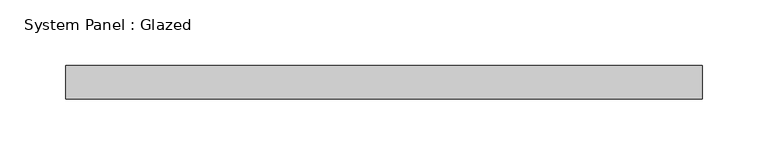
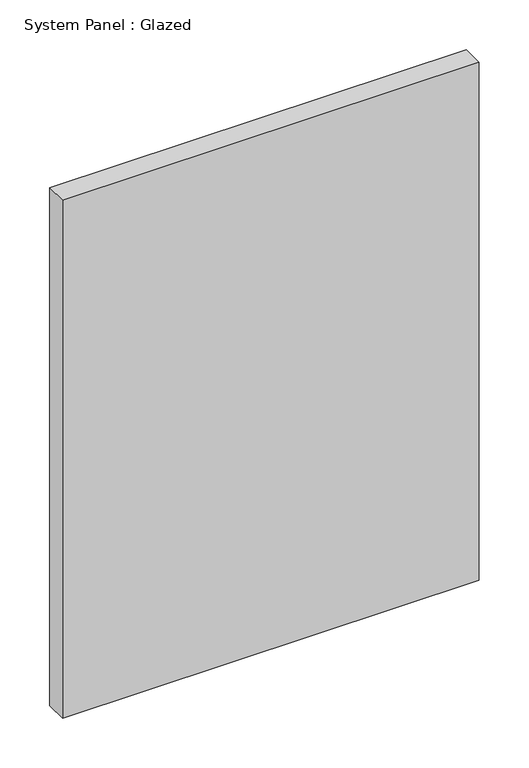
"""IFC4 building model written with IfcOpenShell, lengths in millimetres: plate geometry, System Panel : Glazed."""

from ifc_helpers import new_model, si_unit, origin, origin_with_axes, place, context, project, spatial, polyline, outline, extrude, source, transform, mapped, element, save


def system_panel_glazed_483907af(model_context):
    return source(origin(), model_context, "Body", "SweptSolid", [
        extrude(outline(polyline([(241.3, 19.05), (-241.3, 19.05), (-241.3, 44.45), (241.3, 44.45), (241.3, 19.05)])), origin_with_axes(), (0.0, 0.0, 1.0), 633.9776209),
    ])


if __name__ == "__main__":
    model = new_model("IFC4")
    model_context = context("Model", 3, world=origin())
    ifc_project = project(units=[si_unit("LENGTHUNIT", "METRE", prefix="MILLI")], contexts=[model_context])
    site = spatial("IfcSite", under=ifc_project)
    building = spatial("IfcBuilding", under=site)
    placement = place(None, origin())
    system_panel_glazed_shape = system_panel_glazed_483907af(model_context)
    element("IfcPlate", 1, ObjectType="System Panel : Glazed", at=placement, inside=building, context=model_context, shape_type="MappedRepresentation", body=[
        mapped(system_panel_glazed_shape, transform((0.0, 0.0, 0.0), x_axis=(1.0, 0.0, 0.0), y_axis=(0.0, 1.0, 0.0), z_axis=(0.0, 0.0, 1.0))),
    ])
    save(model, "model.ifc")

# Revit data of these elements
# Type "System Panel : Glazed"
#   Construction Type Id = "GSP4R"
#   Analytic Construction = "1/8 in Pilkington single glazing"
#   Visual Light Transmittance = 0.9
#   Solar Heat Gain Coefficient = 0.86
#   Heat Transfer Coefficient (U) = 1.18115 BTU/(h·ft²·°F)
#   Define Thermal Properties by = 1
# Element 1 (IfcPlate, "System Panel : Glazed")
#   Materials on its faces: "Glass"
# Materials
#   "Glass": class "Glass", colour RGB 0 128 192, transparency 0.75, Description = "Soda Lime Glass", Cost = 0
